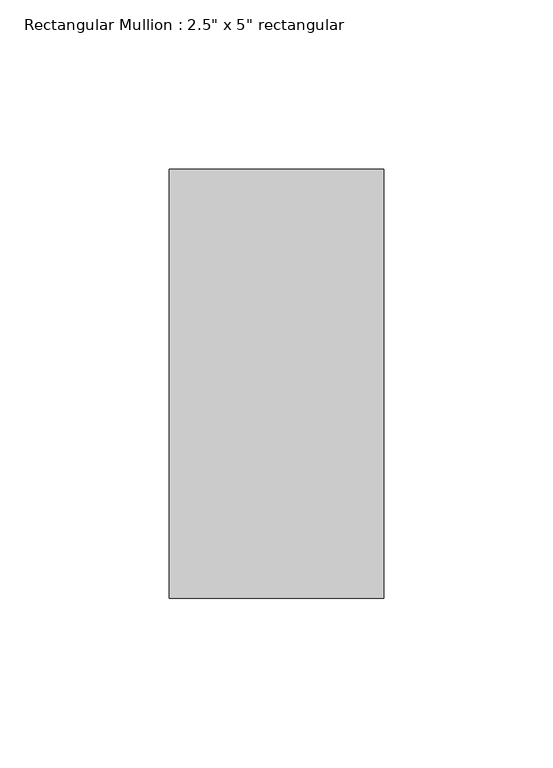
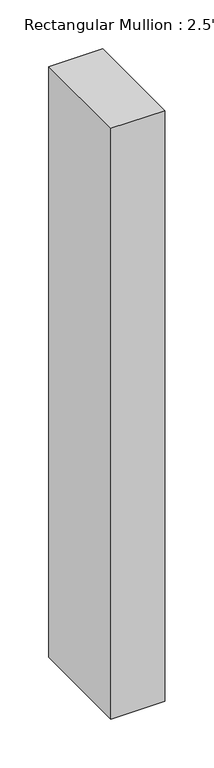
"""IFC4 building model written with IfcOpenShell, lengths in millimetres: member geometry."""

from ifc_helpers import new_model, si_unit, frame, origin, place, context, project, spatial, polyline, outline, extrude, source, transform, mapped, element, save


def member_cae490a4(model_context):
    return source(origin(), model_context, "Body", "SweptSolid", [
        extrude(outline(polyline([(0.0, 63.5), (0.0, -63.5), (-63.5, -63.5), (-63.5, 63.5), (0.0, 63.5)])), frame((0.0, 0.0, -737.3956367), z_axis=(0.0, 0.0, 1.0), x_axis=(1.0, 0.0, 0.0)), (0.0, 0.0, 1.0), 737.3956367),
    ])


if __name__ == "__main__":
    model = new_model("IFC4")
    model_context = context("Model", 3, world=origin())
    ifc_project = project(units=[si_unit("LENGTHUNIT", "METRE", prefix="MILLI")], contexts=[model_context])
    site = spatial("IfcSite", under=ifc_project)
    building = spatial("IfcBuilding", under=site)
    placement = place(None, origin())
    member_shape = member_cae490a4(model_context)
    element("IfcMember", 1, ObjectType="Rectangular Mullion : 2.5\" x 5\" rectangular", at=placement, inside=building, context=model_context, shape_type="MappedRepresentation", body=[
        mapped(member_shape, transform((0.0, 0.0, 0.0), x_axis=(1.0, 0.0, 0.0), y_axis=(0.0, 1.0, 0.0), z_axis=(0.0, 0.0, 1.0))),
    ])
    save(model, "model.ifc")

# Revit data of these elements
# Type "Rectangular Mullion : 2.5\" x 5\" rectangular"
#   built-in parameter 1007304 = 0.416667 (stored number, unit not read)
#   built-in parameter 1007301 = 0.104167 (stored number, unit not read)
#   built-in parameter 1007300 = 0.104167 (stored number, unit not read)
# Element 1 (IfcMember, "Rectangular Mullion : 2.5\" x 5\" rectangular")
#   Materials on its faces: "Aluminum"
# Materials
#   "Aluminum": class "Metal", colour RGB 247 247 247, transparency 0, Description = "Aluminum 6061", Cost = 0
